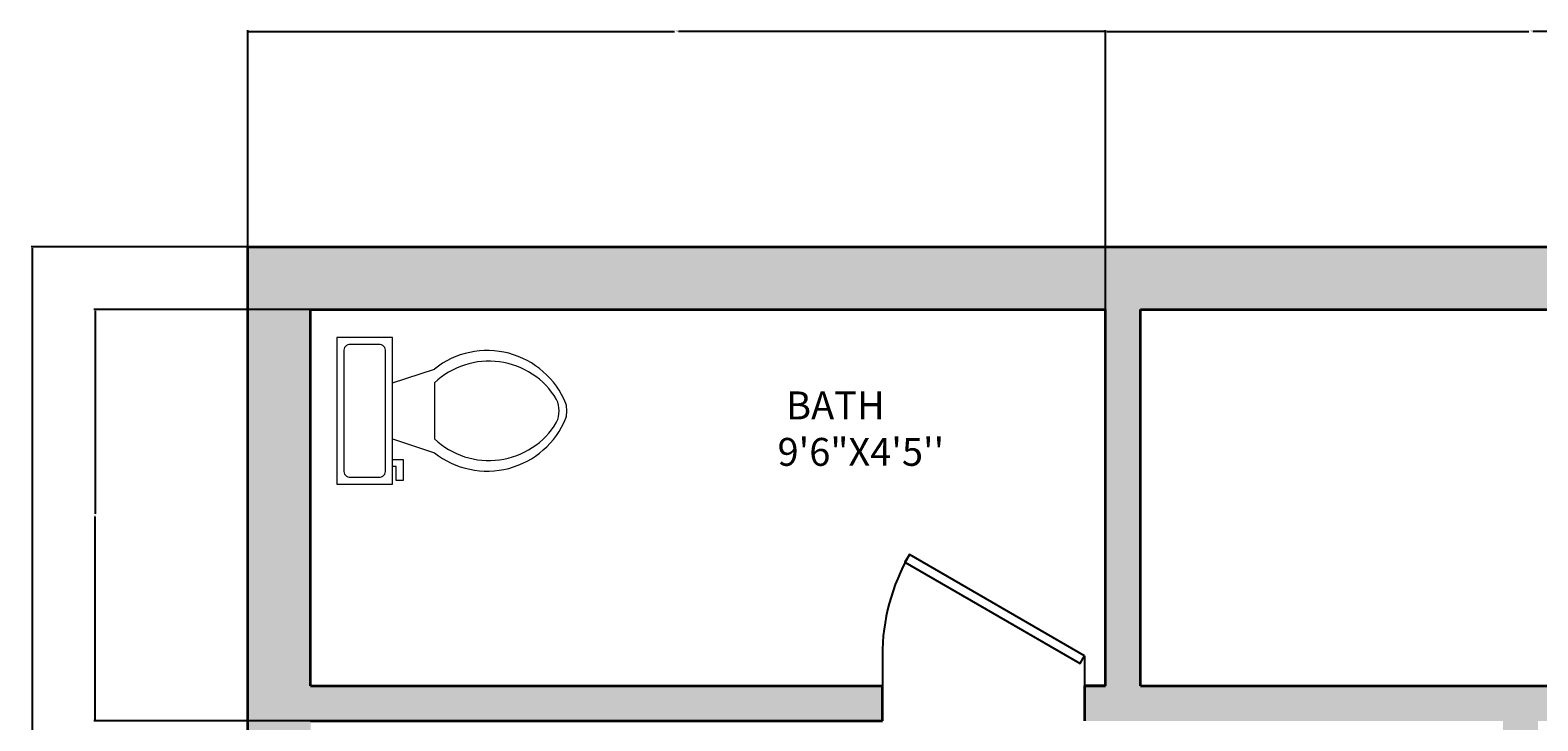
# Model space of a CAD drawing. Units: inches. Extents: x -30 to 437, y -29 to 647.
# Tile 9 of 15: x -30 to 187, y 548 to 647. Entities that reach past the tile are written whole.
import ezdxf

# ---------------------------------------------------------------- set-up
doc = ezdxf.new("R2010")
doc.units = ezdxf.units.IN
doc.header["$MEASUREMENT"] = 0
for name, color, linetype, lineweight in [('A-ANNO-DIMS', 2, 'Continuous', 18), ('A-AREA-IDEN', 7, 'Continuous', 18), ('A-WALL', 7, 'Continuous', 35), ('bathroom', 90, 'Continuous', 18), ('doors', 40, 'Continuous', 25)]:
    doc.layers.add(name, color=color, linetype=linetype, lineweight=lineweight)
doc.layers.add('A-WALL-PATT', color=251, linetype='Continuous', lineweight=13, true_color=0x636466)
doc.styles.get("Standard").update_dxf_attribs({"font": 'arial.ttf'})
doc.dimstyles.get("Standard").update_dxf_attribs({"dimtxt": 0.18, "dimasz": 0.18, "dimexe": 0.18, "dimexo": 0.0625, "dimgap": 0.09, "dimtad": 0, "dimtih": 1, "dimtoh": 1, "dimdec": 4, "dimzin": 0, "dimdsep": 46, "dimtxsty": 'Standard', "dimcen": 0.09, "dimadec": 0, "dimazin": 0, "dimtfac": 1, "dimtdec": 4, "dimtofl": 0, "dimtmove": 0, "dimatfit": 3, "dimfxl": 1, "dimtolj": 1, "dimtzin": 0, "dimarcsym": 0})

# ---------------------------------------------------------------- blocks, each defined once
blk = doc.blocks.new('Toilet - top')
for p, q in [((9.5, -6), (9.5, -2)), ((-10, -8.5), (-8, -8.5)), ((-10, -9.5), (-10, -8.5)), ((-8, -8.5), (-8, -8)), ((-7, -8), (-7, -9.5)), ((-4, -8), (-6, -14)), ((4, -8), (6, -14)), ((-7, -9.5), (-10, -9.5)), ((4, -14), (-4, -14))]:
    blk.add_line(p, q)
blk.add_lwpolyline([(10.5, -8), (10.5, 0), (-10.5, 0), (-10.5, -8)], close=True)
for points in [[(-9.5, -2), (-9.5, -6)], [(8.5, -1), (-8.5, -1)], [(-8.5, -7), (8.5, -7)]]:
    blk.add_lwpolyline(points)
for centre, radius, start, end in [((-8.62, -1.88), 0.884, 81.8699, 188.1301), ((8.62, -1.88), 0.884, 351.8699, 98.1301), ((-8.62, -6.12), 0.884, 171.8699, 278.1301), ((8.62, -6.12), 0.884, 261.8699, 8.1301), ((3.52, -21.58), 12.17, 141.4691, 247.9714), ((4.2, -21.82), 11.33, 136.3677, 238.9468), ((-3.52, -21.58), 12.17, 292.0284, 38.5307), ((-4.2, -21.82), 11.33, 301.053, 43.6321), ((0, -27.88), 4, 245.7318, 294.2682), ((0, -29), 4, 254.8605, 285.1395)]:
    blk.add_arc(centre, radius, start, end)
blk = doc.blocks.new('*U7')
for p, q in [((0, 0), (0, 6)), ((40, 0), (40, 6))]:
    blk.add_line(p, q)
blk.add_lwpolyline([(0, 0), (34.64, -20), (35.52, -18.48), (0.87, 1.52)], close=True)
blk.add_arc((0, 0), 40, 330, 0)
blk = doc.blocks.new('*D26')
at = {"layer": 'A-ANNO-DIMS', "color": 0, "lineweight": -2, "transparency": 16777216}
for p, q in [((1.61, 615.55), (-29.41, 615.55)), ((-29.23, 615.37), (-29.23, 308.98)), ((-29.23, 2.23), (-29.23, 308.62)), ((1.61, 2.05), (-29.41, 2.05))]:
    blk.add_line(p, q, dxfattribs=at)
at = {"layer": 'A-ANNO-DIMS', "color": 0, "transparency": 16777216}
for points in [[(-29.26, 615.37), (-29.2, 615.37), (-29.23, 615.55)], [(-29.26, 2.23), (-29.2, 2.23), (-29.23, 2.05)]]:
    blk.add_solid(points, dxfattribs=at)
at = {"layer": 'Defpoints', "color": 0, "transparency": 16777216}
for p in [(-29.23, 615.55), (1.67, 615.55), (1.67, 2.05)]:
    blk.add_point(p, dxfattribs=at)
at = {"layer": 'A-ANNO-DIMS', "color": 0, "transparency": 16777216, "insert": (-29.23, 308.8), "char_height": 0.18, "attachment_point": 5}
blk.add_mtext('\\A1;613.5', dxfattribs=at)
blk = doc.blocks.new('*D27')
at = {"layer": 'A-ANNO-DIMS', "color": 0, "lineweight": -2, "transparency": 16777216}
for p, q in [((1.67, 615.61), (1.67, 646.63)), ((124.67, 606.61), (124.67, 646.63)), ((1.85, 646.45), (62.89, 646.45)), ((124.49, 646.45), (63.45, 646.45))]:
    blk.add_line(p, q, dxfattribs=at)
at = {"layer": 'A-ANNO-DIMS', "color": 0, "transparency": 16777216}
for points in [[(1.85, 646.48), (1.85, 646.42), (1.67, 646.45)], [(124.49, 646.48), (124.49, 646.42), (124.67, 646.45)]]:
    blk.add_solid(points, dxfattribs=at)
at = {"layer": 'Defpoints', "color": 0, "transparency": 16777216}
for p in [(124.67, 646.45), (1.67, 615.55), (124.67, 606.55)]:
    blk.add_point(p, dxfattribs=at)
at = {"layer": 'A-ANNO-DIMS', "color": 0, "transparency": 16777216, "insert": (63.17, 646.45), "char_height": 0.18, "attachment_point": 5}
blk.add_mtext('\\A1;123', dxfattribs=at)
blk = doc.blocks.new('*D28')
at = {"layer": 'A-ANNO-DIMS', "color": 0, "lineweight": -2, "transparency": 16777216}
for p, q in [((124.67, 606.61), (124.67, 646.63)), ((246.67, 606.61), (246.67, 646.63)), ((124.85, 646.45), (185.39, 646.45)), ((246.49, 646.45), (185.95, 646.45))]:
    blk.add_line(p, q, dxfattribs=at)
at = {"layer": 'A-ANNO-DIMS', "color": 0, "transparency": 16777216}
for points in [[(124.85, 646.48), (124.85, 646.42), (124.67, 646.45)], [(246.49, 646.48), (246.49, 646.42), (246.67, 646.45)]]:
    blk.add_solid(points, dxfattribs=at)
at = {"layer": 'Defpoints', "color": 0, "transparency": 16777216}
for p in [(246.67, 646.45), (124.67, 606.55), (246.67, 606.55)]:
    blk.add_point(p, dxfattribs=at)
at = {"layer": 'A-ANNO-DIMS', "color": 0, "transparency": 16777216, "insert": (185.67, 646.45), "char_height": 0.18, "attachment_point": 5}
blk.add_mtext('\\A1;122', dxfattribs=at)
blk = doc.blocks.new('*D34')
at = {"layer": 'A-ANNO-DIMS', "color": 0, "lineweight": -2, "transparency": 16777216}
for p, q in [((10.61, 606.55), (-20.41, 606.55)), ((-20.23, 606.37), (-20.23, 577.23)), ((-20.23, 547.73), (-20.23, 576.87)), ((10.61, 547.55), (-20.41, 547.55))]:
    blk.add_line(p, q, dxfattribs=at)
at = {"layer": 'A-ANNO-DIMS', "color": 0, "transparency": 16777216}
for points in [[(-20.26, 606.37), (-20.2, 606.37), (-20.23, 606.55)], [(-20.26, 547.73), (-20.2, 547.73), (-20.23, 547.55)]]:
    blk.add_solid(points, dxfattribs=at)
at = {"layer": 'Defpoints', "color": 0, "transparency": 16777216}
for p in [(-20.23, 606.55), (10.67, 606.55), (10.67, 547.55)]:
    blk.add_point(p, dxfattribs=at)
at = {"layer": 'A-ANNO-DIMS', "color": 0, "transparency": 16777216, "insert": (-20.23, 577.05), "char_height": 0.18, "attachment_point": 5}
blk.add_mtext('\\A1;59', dxfattribs=at)

msp = doc.modelspace()

# ---------------------------------------------------------------- hatches: boundary and pattern name
at = {"layer": 'A-WALL-PATT'}
h = msp.add_hatch(color=256, dxfattribs=at)
h.dxf.hatch_style = 1
h.paths.add_polyline_path([(393.6054, 183.2352), (369.6054, 183.2352), (369.6054, 213.2352), (393.6054, 213.2352), (393.6054, 207.2352), (394.6054, 207.2352), (394.6054, 211.2352), (395.6054, 211.2352), (395.6054, 185.2352), (394.6054, 185.2352), (394.6054, 189.2352), (393.6054, 189.2352)], flags=0)
h.paths.add_polyline_path([(384.6054, 189.2352, -1), (390.6054, 189.2352, -1)], flags=0)
h.paths.add_polyline_path([(385.6054, 189.2352, -1), (389.6054, 189.2352, -1)], flags=0)
h.paths.add_polyline_path([(374.6054, 189.2352, -1), (382.6054, 189.2352, -1)], flags=0)
h.paths.add_polyline_path([(386.6054, 189.2352, -1), (388.6054, 189.2352, -1)], flags=0)
h.paths.add_polyline_path([(375.6054, 189.2352, -1), (381.6054, 189.2352, -1)], flags=0)
h.paths.add_polyline_path([(376.6054, 189.2352, -1), (380.6054, 189.2352, -1)], flags=0)
h.paths.add_polyline_path([(377.6054, 189.2352, -1), (379.6054, 189.2352, -1)], flags=0)
h.paths.add_polyline_path([(390.6054, 195.2352), (374.6054, 195.2352), (374.6054, 201.2352), (390.6054, 201.2352)], flags=0)
h.paths.add_polyline_path([(389.6054, 196.2352), (375.6054, 196.2352), (375.6054, 200.2352), (389.6054, 200.2352)], flags=0)
h.paths.add_polyline_path([(383.6054, 207.2352, -1), (391.6054, 207.2352, -1)], flags=0)
h.paths.add_polyline_path([(384.6054, 207.2352, -1), (390.6054, 207.2352, -1)], flags=0)
h.paths.add_polyline_path([(385.6054, 207.2352, -1), (389.6054, 207.2352, -1)], flags=0)
h.paths.add_polyline_path([(386.6054, 207.2352, -1), (388.6054, 207.2352, -1)], flags=0)
h.paths.add_polyline_path([(375.6054, 207.2352, -1), (381.6054, 207.2352, -1)], flags=0)
h.paths.add_polyline_path([(376.6054, 207.2352, -1), (380.6054, 207.2352, -1)], flags=0)
h.paths.add_polyline_path([(377.6054, 207.2352, -1), (379.6054, 207.2352, -1)], flags=0)
h.paths.add_polyline_path([(305.5437, 160.3663, -0.41421356), (304.0437, 158.8663), (271.0437, 158.8663, -0.41421356), (269.5437, 160.3663), (269.5437, 178.3663, -0.41421356), (271.0437, 179.8663), (304.0437, 179.8663, -0.41421356), (305.5437, 178.3663)], flags=0)
h.paths.add_polyline_path([(304.0437, 165.3663, -0.41421356), (303.0437, 164.3663), (289.2937, 164.3663, -0.41421356), (288.2937, 165.3663), (288.2937, 177.3663, -0.41421356), (289.2937, 178.3663), (303.0437, 178.3663, -0.41421356), (304.0437, 177.3663)], flags=0)
h.paths.add_polyline_path([(296.5437, 171.3663, -1), (295.5437, 171.3663, -1)], flags=0)
h.paths.add_polyline_path([(286.7937, 165.3663, -0.41421356), (285.7937, 164.3663), (272.0437, 164.3663, -0.41421356), (271.0437, 165.3663), (271.0437, 177.3663, -0.41421356), (272.0437, 178.3663), (285.7937, 178.3663, -0.41421356), (286.7937, 177.3663)], flags=0)
h.paths.add_polyline_path([(279.5437, 171.3663, -1), (278.5437, 171.3663, -1)], flags=0)
h.paths.add_polyline_path([(360.6737, 290.5474), (360.6737, 300.5474), (396.6737, 300.5474), (396.6737, 290.5474)], flags=0)
h.paths.add_polyline_path([(259.6737, 124.5474), (259.6737, 114.5474), (171.6737, 114.5474), (171.6737, 124.5474)], flags=0)
h.paths.add_polyline_path([(288.0737, 215.3705), (286.7097, 214.583), (268.7097, 245.7599), (270.0737, 246.5474)], flags=0)
h.paths.add_polyline_path([(259.6737, 168.5474), (256.6737, 168.5474), (256.6737, 173.5474), (256.6737, 179.0224), (255.8753, 177.6395), (224.2956, 195.872, 0.12053744), (220.1737, 179.0224, 0.12053744), (216.0518, 195.872), (184.4721, 177.6395), (183.6737, 179.0224), (215.2836, 197.2724), (216.0821, 195.8895), (216.0518, 195.872, -0.12053744), (220.1737, 179.0224, -0.12053744), (224.2956, 195.872), (224.2653, 195.8895), (225.0638, 197.2724), (256.6737, 179.0224), (256.6737, 173.5474), (259.6737, 173.5474)], flags=0)
h.paths.add_polyline_path([(386.7943, 325.4601), (372.6871, 325.4601), (372.6871, 339.5673), (386.7943, 339.5673)], flags=0)
h.paths.add_polyline_path([(359.5875, 343.7429), (357.7905, 343.7429), (357.7905, 327.9179), (359.3933, 327.9179, 0.41420885), (361.5302, 330.0549), (361.5302, 341.8434, 0.41436161)], flags=0)
h.paths.add_polyline_path([(341.7887, 323.1235, -0.11921667), (340.7839, 323.1235)], flags=0)
h.paths.add_polyline_path([(379.6332, 328.8632), (379.6332, 332.2699), (376.0992, 332.2699, 0.39427733)], flags=0)
h.paths.add_polyline_path([(375.5299, 332.459, -1), (383.8511, 332.459, -1)], flags=0)
h.paths.add_polyline_path([(388.9363, 344.7425), (372.5309, 344.7425, -0.41421356), (370.394, 346.8794), (370.394, 347.5594, -0.39085173), (372.3472, 349.7005, -0.43951011), (370.394, 351.4933), (370.394, 365.1894, -0.40305452), (372.2191, 367.1298, -0.41839453), (370.394, 368.9291), (370.394, 382.6251, -0.40885826), (372.2519, 384.5722, -0.42377324), (370.394, 386.3707), (370.394, 400.0667, -0.38660687), (372.1327, 402.0094), (372.531, 402.0094, -0.41421834), (370.394, 404.1464), (370.394, 404.7778, -0.41420891), (372.5309, 406.9147), (388.9363, 406.9147, -0.41421821), (391.0733, 404.7778), (391.0733, 346.8794, -0.41421356)], flags=0)
edge = h.paths.add_edge_path(flags=0)
edge.add_spline(control_points=[(349.3585, 363.204), (349.0859, 363.204), (348.8133, 363.2227), (348.2712, 363.2973), (348.0016, 363.3531), (347.3533, 363.5328), (346.9776, 363.6755), (346.2445, 364.0308), (345.887, 364.2432), (345.1953, 364.7329), (344.8611, 365.0101), (344.2197, 365.6237), (343.9125, 365.9603), (343.211, 366.8336), (342.8313, 367.3965), (342.1401, 368.6117), (341.8286, 369.2641), (341.2807, 370.64), (341.0443, 371.3636), (340.6522, 372.8619), (340.4964, 373.6367), (340.2695, 375.2158), (340.1983, 376.0203), (340.142, 377.6365), (340.157, 378.4483), (340.2729, 380.0567), (340.3738, 380.8533), (340.6589, 382.4093), (340.8432, 383.1686), (341.2906, 384.629), (341.5538, 385.3301), (342.1531, 386.6544), (342.4891, 387.2776), (343.2266, 388.4288), (343.6281, 388.9567), (344.4879, 389.9012), (344.9463, 390.3178), (345.7981, 390.9428), (346.182, 391.1771), (346.9712, 391.5648), (347.3766, 391.7182), (348.2004, 391.9387), (348.6189, 392.0058), (349.4588, 392.0508), (349.8801, 392.0288), (350.7146, 391.8966), (351.1278, 391.7865), (351.9366, 391.4822), (352.3323, 391.2882), (353.0989, 390.8223), (353.4699, 390.5504), (354.1819, 389.9355), (354.5229, 389.5924), (355.1706, 388.8418), (355.4772, 388.4343), (356.1315, 387.4422), (356.4671, 386.8397), (357.0692, 385.5581), (357.3356, 384.879), (357.7933, 383.4624), (357.9846, 382.725), (358.2875, 381.2112), (358.3992, 380.4349), (358.5404, 378.8643), (358.5699, 378.0699), (358.546, 376.4841), (358.4926, 375.6928), (358.3042, 374.1343), (358.1692, 373.3672), (357.8207, 371.8774), (357.6072, 371.1549), (357.1067, 369.7735), (356.8196, 369.1148), (356.1782, 367.8787), (355.8238, 367.3013), (355.0551, 366.244), (354.6408, 365.7641), (353.7607, 364.9161), (353.2948, 364.5481), (352.445, 364.0149), (352.0701, 363.822), (351.3034, 363.5117), (350.9116, 363.3943), (350.1325, 363.2418), (349.7455, 363.204), (349.3585, 363.204)], knot_values=[3.14159265, 3.14159265, 3.14159265, 3.14159265, 3.22691715, 3.22691715, 3.31224165, 3.31224165, 3.43426671, 3.43426671, 3.55629177, 3.55629177, 3.67831683, 3.67831683, 3.8003419, 3.8003419, 3.97157384, 3.97157384, 4.14280577, 4.14280577, 4.31403771, 4.31403771, 4.48526965, 4.48526965, 4.65650159, 4.65650159, 4.82773353, 4.82773353, 4.99896547, 4.99896547, 5.1701974, 5.1701974, 5.34142934, 5.34142934, 5.51266128, 5.51266128, 5.68389322, 5.68389322, 5.85512516, 5.85512516, 5.98669107, 5.98669107, 6.11825699, 6.11825699, 6.24982291, 6.24982291, 6.38138882, 6.38138882, 6.51295474, 6.51295474, 6.64452065, 6.64452065, 6.77608657, 6.77608657, 6.90765249, 6.90765249, 7.0392184, 7.0392184, 7.20701563, 7.20701563, 7.37481286, 7.37481286, 7.54261009, 7.54261009, 7.71040732, 7.71040732, 7.87820455, 7.87820455, 8.04600178, 8.04600178, 8.21379901, 8.21379901, 8.38159624, 8.38159624, 8.54939347, 8.54939347, 8.7171907, 8.7171907, 8.88498794, 8.88498794, 9.05278517, 9.05278517, 9.17820699, 9.17820699, 9.30362881, 9.30362881, 9.42477796, 9.42477796, 9.42477796, 9.42477796], degree=3, periodic=0)
edge.add_line((341.1696, 384.3006), (341.2012, 384.2808))
edge = h.paths.add_edge_path(flags=0)
edge.add_line((344.3353, 388.7801), (344.317, 388.7915))
edge.add_ellipse((349.3585, 377.6204), major_axis=(0, -13.7895), ratio=0.62186025, start_angle=-244.867444, end_angle=-124.769923)
h.paths.add_polyline_path([(163.6737, 163.1474), (132.4968, 145.1474), (131.7093, 146.5114), (162.8862, 164.5114)], flags=0)
h.paths.add_polyline_path([(366.4355, 409.0896, -0.41423669), (364.2985, 406.9525, -0.4913499), (361.5302, 408.8973), (361.5302, 420.6405, 0.41421356), (359.3932, 422.7775), (357.7905, 422.7775), (357.7905, 406.9525), (359.6317, 406.9525, 0.42741026), (361.5332, 408.9757, 0.39869469), (363.6672, 406.9525, 0.51958103), (366.4355, 409.0895)], flags=0)
h.paths.add_polyline_path([(386.7943, 410.9671), (372.6871, 410.9671), (372.6871, 425.0742), (386.7943, 425.0742)], flags=0)
h.paths.add_polyline_path([(379.6332, 414.3701), (379.6332, 417.7768), (376.0992, 417.7768, 0.39427733)], flags=0)
h.paths.add_polyline_path([(375.5299, 417.966, -1), (383.8511, 417.966, -1)], flags=0)
h.paths.add_polyline_path([(150.0377, 351.583), (148.6737, 352.3705), (166.6737, 383.5474), (168.0377, 382.7599)], flags=0)
h.paths.add_polyline_path([(91.6737, 234.1974), (66.559, 219.6974), (65.9246, 220.7962), (91.0393, 235.2962)], flags=0)
h.paths.add_polyline_path([(255.4612, 443.5834), (254.6737, 444.9474), (285.8506, 462.9474), (286.6381, 461.5834)], flags=0)
h.paths.add_polyline_path([(176.2737, 394.5474), (158.2737, 425.7243), (159.6377, 426.5118), (177.6377, 395.3349)], flags=0)
h.paths.add_polyline_path([(243.6737, 439.5474), (243.0393, 438.4486), (217.9246, 452.9486), (218.559, 454.0474)], flags=0)
h.paths.add_polyline_path([(38.1264, 269.8429), (40.2408, 269.8429), (40.2408, 270.3508), (38.1264, 270.3508)], flags=0)
h.paths.add_polyline_path([(75.7157, 289.9439), (40.2408, 289.9439), (38.1264, 289.6524), (40.2408, 289.6524)], flags=0)
h.paths.add_polyline_path([(75.7157, 270.0846), (77.6447, 270.0846), (77.6697, 270.1626), (75.7175, 270.1626)], flags=0)
h.paths.add_polyline_path([(80.5373, 293.3002), (33.0467, 293.3002), (13.5054, 293.3002), (13.5054, 351.9244), (29.7898, 351.9244), (80.5373, 351.9244)], flags=0)
h.paths.add_polyline_path([(46.0261, 212.466, -0.50131678), (27.1651, 207.5106), (21.165, 209.5107), (21.165, 206.5107), (22.665, 206.5107), (22.665, 203.5107), (21.165, 203.5107), (21.165, 203.0107), (13.165, 203.0107), (13.165, 224.0107), (21.165, 224.0107), (21.165, 217.5107), (27.1649, 219.5106, -0.50132349), (46.0261, 214.5554, -0.13289091)], flags=0)
h.paths.add_polyline_path([(44.688, 211.8666, -0.48007965), (27.165, 209.5107), (27.165, 217.5107, -0.4800795), (44.688, 215.1547, -0.21500378)], flags=0)
h.paths.add_polyline_path([(19.415, 204.0107), (15.165, 204.0107, -0.41421356), (14.165, 204.7607), (14.165, 222.0107, -0.41421356), (14.915, 223.0107), (19.165, 223.0107, -0.41421356), (20.165, 222.2607), (20.165, 205.0107, -0.41421356)], flags=0)
h.paths.add_polyline_path([(32.7608, 269.0719), (31.8439, 269.0719), (31.8439, 268.6134), (13.5054, 268.6134), (13.5054, 291.5366), (31.8439, 291.5366), (32.7608, 291.0781), (32.7608, 280.9919, -1), (32.7608, 279.1581)], flags=0)
h.paths.add_polyline_path([(40.2408, 360.1436), (38.1264, 360.1436), (38.1264, 359.6357), (40.2408, 359.6357)], flags=0)
h.paths.add_polyline_path([(75.7157, 355.2807), (40.2408, 355.2807), (38.1264, 355.5722), (40.2408, 355.5722), (40.2408, 355.2807), (75.7157, 355.2807), (75.7157, 375.5982), (40.2408, 375.5982), (38.1264, 375.3817), (40.2408, 375.3817), (40.2408, 375.5982), (75.7157, 375.5982), (77.9733, 375.062), (75.7175, 375.062), (75.7175, 374.554)], flags=0)
h.paths.add_polyline_path([(42.8174, 299.814, 0.13867074), (34.1602, 294.603), (14.8081, 294.603), (14.8081, 350.6216), (29.8539, 350.6216, 0.09822056)], flags=0)
h.paths.add_polyline_path([(15.8636, 276.7781, -0.30640166), (20.3757, 283.4499), (20.3483, 290.6726), (31.4014, 290.7146), (31.4309, 282.9124), (26.8287, 282.895, -0.26006276), (30.241, 276.7781, -1)], flags=0)
h.paths.add_polyline_path([(26.1332, 276.7781), (23.0523, 273.6972), (19.9714, 276.7781), (23.0523, 279.8589), (23.0523, 283.9209), (21.3493, 283.9145), (20.7006, 283.5219), (20.6907, 286.1226), (23.2914, 286.1325), (25.8936, 285.7522), (27.1939, 285.7572), (28.4928, 286.1522), (31.0935, 286.1621), (31.0918, 286.6172), (25.6303, 286.5965), (25.616, 290.3675), (31.0775, 290.3882), (31.0918, 286.6172), (31.1034, 283.5614), (28.5027, 283.5515), (25.9005, 283.9317), (23.0523, 283.9209), (23.0523, 279.8589)], flags=0)
h.paths.add_polyline_path([(24.0793, 276.7781, -1), (22.0253, 276.7781, -1)], flags=0)
h.paths.add_polyline_path([(35.7687, 302.2895, -0.41421356), (35.2283, 301.2726), (22.2164, 297.2909, -0.41421356), (21.1995, 297.8313), (15.7317, 315.6996, -0.41421356), (16.2721, 316.7165), (18.8554, 317.507), (15.3721, 328.8904, -0.41421356), (15.9125, 329.9073), (28.9244, 333.889, -0.41421356), (29.9414, 333.3486), (35.4091, 315.4802, -0.41421356), (34.8687, 314.4633), (32.2854, 313.6728)], flags=0)
h.paths.add_polyline_path([(361.3728, 532.6207), (302.7487, 532.6207), (302.7487, 580.1113), (302.7487, 599.6527), (361.3728, 599.6527), (361.3728, 583.3682)], flags=0)
h.paths.add_polyline_path([(370.1, 575.0316), (370.1, 572.9172), (370.6079, 572.9172), (370.6079, 575.0316)], flags=0)
h.paths.add_polyline_path([(385.0466, 537.4423), (385.0466, 572.9172), (384.8302, 575.0316), (384.8302, 572.9172)], flags=0)
h.paths.add_polyline_path([(384.5104, 535.3262), (384.5104, 537.4406), (384.0025, 537.4406), (364.7291, 537.4423), (364.7291, 572.9172), (365.0206, 575.0316), (365.0206, 572.9172), (364.7291, 572.9172), (364.7291, 537.4423), (384.5884, 537.4423), (384.5884, 535.5133)], flags=0)
h.paths.add_polyline_path([(384.5884, 535.5133), (383.4945, 535.164), (383.4945, 537.4406), (382.9866, 535.3262), (382.9866, 537.4406), (383.4945, 535.3262), (383.4945, 537.4406), (384.5884, 537.4406)], flags=0)
h.paths.add_polyline_path([(23.874, 286.8174), (21.0132, 286.8065), (21.0004, 290.1875), (23.8612, 290.1983)], flags=0)
h.paths.add_polyline_path([(242.9824, 511.1667), (234.9824, 511.1667), (234.9824, 517.6667), (228.9825, 515.6667, -0.50132349), (210.1213, 520.622, -0.13289091), (210.1213, 522.7114, -0.50131678), (228.9823, 527.6667), (234.9824, 525.6667), (234.9824, 528.6667), (233.4824, 528.6667), (233.4824, 531.6667), (234.9824, 531.6667), (234.9824, 532.1667), (242.9824, 532.1667)], flags=0)
h.paths.add_polyline_path([(236.9824, 512.1667, -0.41421356), (235.9824, 512.9167), (235.9824, 530.1667, -0.41421356), (236.7324, 531.1667), (240.9824, 531.1667, -0.41421356), (241.9824, 530.4167), (241.9824, 513.1667, -0.41421356), (241.2324, 512.1667)], flags=0)
h.paths.add_polyline_path([(279.533, 537.4423), (279.533, 535.5133), (279.6111, 535.4884), (279.6111, 537.4406)], flags=0)
h.paths.add_polyline_path([(279.2913, 575.0316), (279.2913, 572.9172), (279.7992, 572.9172), (279.7992, 575.0316)], flags=0)
h.paths.add_polyline_path([(211.4594, 520.0227, -0.21500378), (211.4594, 523.3107, -0.48007965), (228.9824, 525.6667), (228.9824, 517.6667, -0.4800795)], flags=0)
h.paths.add_polyline_path([(32.7627, 354.1465), (31.8457, 354.1465), (31.8457, 353.688), (13.5054, 353.688), (13.5054, 376.6134), (31.8457, 376.6134), (32.7627, 376.1549), (32.7627, 366.0677, -1), (32.7627, 364.2337)], flags=0)
h.paths.add_polyline_path([(15.9446, 365.1507, -1), (30.3234, 365.1507, -1)], flags=0)
h.paths.add_polyline_path([(41.213, 428.467), (43.3274, 428.467), (43.3274, 428.9749), (41.213, 428.9749)], flags=0)
h.paths.add_polyline_path([(78.8022, 448.568), (43.3274, 448.568), (41.213, 448.2765), (43.3274, 448.2765)], flags=0)
h.paths.add_polyline_path([(78.8022, 428.7087), (80.7313, 428.7087), (80.7562, 428.7868), (78.804, 428.7868)], flags=0)
h.paths.add_polyline_path([(26.2152, 365.1507), (23.134, 362.0696), (20.0529, 365.1507), (23.134, 368.2319)], flags=0)
h.paths.add_polyline_path([(24.1611, 365.1507, -1), (22.107, 365.1507, -1)], flags=0)
h.paths.add_polyline_path([(309.2625, 570.3406, 0.13867074), (304.0514, 578.9978), (304.0514, 598.3499), (360.07, 598.3499), (360.07, 583.3041, 0.09822056)], flags=0)
h.paths.add_polyline_path([(246.6737, 552.5474), (129.6737, 552.5474), (129.6737, 606.5474), (246.6737, 606.5474)], flags=16)
h.paths.add_polyline_path([(373.6822, 580.3953), (363.595, 580.3953), (363.595, 581.3123), (363.1365, 581.3123), (363.1365, 599.6527), (386.0619, 599.6527), (386.0619, 581.3123), (385.6034, 580.3953), (375.5162, 580.3953, -1)], flags=0)
h.paths.add_polyline_path([(83.6239, 451.9244), (36.1333, 451.9244), (16.5919, 451.9244), (16.5919, 510.5485), (32.8764, 510.5485), (83.6239, 510.5485)], flags=0)
h.paths.add_polyline_path([(367.4098, 590.024, -1), (381.7886, 590.024, -1)], flags=0)
h.paths.add_polyline_path([(374.5992, 586.9428), (371.518, 590.024), (374.5992, 593.1052), (377.6803, 590.024)], flags=0)
h.paths.add_polyline_path([(373.5721, 590.024, -1), (375.6262, 590.024, -1)], flags=0)
h.paths.add_polyline_path([(324.9287, 577.7489, -0.41421356), (323.9118, 578.2893), (323.1212, 580.8726), (311.7379, 577.3893, -0.41421356), (310.721, 577.9297), (306.7393, 590.9416, -0.41421356), (307.2797, 591.9585), (325.1481, 597.4263, -0.41421356), (326.165, 596.8859), (326.9555, 594.3026), (338.3388, 597.7859, -0.41421356), (339.3557, 597.2455), (343.3374, 584.2336, -0.41421356), (342.797, 583.2167)], flags=0)
h.paths.add_polyline_path([(300.5265, 580.3972), (290.4404, 580.3972, -1), (288.6065, 580.3972), (278.5203, 580.3972), (278.5203, 581.3142), (278.0619, 581.3142), (278.0619, 599.6527), (300.985, 599.6527), (300.985, 581.3142)], flags=0)
h.paths.add_polyline_path([(300.163, 581.7567), (292.3609, 581.7271), (292.3434, 586.3294, -0.75567924), (279.0378, 590.1057, -0.82536731), (292.8983, 592.7823), (300.1211, 592.8097)], flags=0)
h.paths.add_polyline_path([(299.8367, 582.0805), (296.0656, 582.0662), (293.0098, 582.0546), (292.9999, 584.6553), (293.3802, 587.2575), (293.3694, 590.1057), (289.3074, 590.1057), (286.2265, 587.0248), (283.1456, 590.1057), (286.2265, 593.1866), (289.3074, 590.1057), (293.3694, 590.1057), (293.3629, 591.8088), (292.9703, 592.4575), (295.5711, 592.4673), (295.5809, 589.8666), (295.2007, 587.2644), (295.2056, 585.9641), (295.6006, 584.6652), (295.6105, 582.0645), (296.0656, 582.0662), (296.0449, 587.5277), (299.8159, 587.542)], flags=0)
h.paths.add_polyline_path([(285.1995, 590.1057, -1), (287.2535, 590.1057, -1)], flags=0)
h.paths.add_polyline_path([(299.6467, 589.2969), (296.2658, 589.284), (296.255, 592.1448), (299.6359, 592.1576)], flags=0)
h.paths.add_polyline_path([(35.8473, 427.696), (34.9304, 427.696), (34.9304, 427.2376), (16.5919, 427.2376), (16.5919, 450.1607), (34.9304, 450.1607), (35.8473, 449.7022), (35.8473, 439.6161, -1), (35.8473, 437.7822)], flags=0)
h.paths.add_polyline_path([(18.9502, 435.4022, -0.30640166), (23.4623, 442.074), (23.4349, 449.2968), (34.4879, 449.3387), (34.5175, 441.5366), (29.9152, 441.5191, -0.26006276), (33.3275, 435.4022, -1)], flags=0)
h.paths.add_polyline_path([(29.2197, 435.4022), (26.1389, 432.3213), (23.058, 435.4022), (26.1389, 438.4831), (26.1389, 442.5451), (24.4358, 442.5386), (23.7871, 442.1461), (23.7772, 444.7468), (26.378, 444.7566), (28.9801, 444.3764), (30.2805, 444.3813), (31.5794, 444.7764), (34.1801, 444.7862), (34.1784, 445.2413), (28.7169, 445.2206), (28.7026, 448.9917), (34.164, 449.0124), (34.1784, 445.2413), (34.1899, 442.1855), (31.5892, 442.1756), (28.987, 442.5559), (26.1389, 442.5451), (26.1389, 438.4831)], flags=0)
h.paths.add_polyline_path([(27.1658, 435.4022, -1), (25.1119, 435.4022, -1)], flags=0)
h.paths.add_polyline_path([(45.904, 458.4382, 0.13867074), (37.2467, 453.2271), (17.8947, 453.2271), (17.8947, 509.2457), (32.9405, 509.2457, 0.09822056)], flags=0)
h.paths.add_polyline_path([(26.9605, 445.4415), (24.0997, 445.4307), (24.0869, 448.8116), (26.9477, 448.8225)], flags=0)
h.paths.add_polyline_path([(38.3149, 459.8967), (25.3029, 455.915, -0.41421356), (24.286, 456.4554), (18.8183, 474.3238, -0.41421356), (19.3586, 475.3407), (21.942, 476.1312), (18.4587, 487.5145, -0.41421356), (18.999, 488.5314), (32.011, 492.5131, -0.41421356), (33.0279, 491.9727), (38.4957, 474.1044, -0.41421356), (37.9553, 473.0875), (35.3719, 472.297), (38.8553, 460.9136, -0.41421356)], flags=0)
h.paths.add_polyline_path([(43.3274, 518.7678), (41.213, 518.7678), (41.213, 518.2598), (43.3274, 518.2598)], flags=0)
h.paths.add_polyline_path([(78.8022, 513.9049), (43.3274, 513.9049), (41.213, 514.1964), (43.3274, 514.1964), (43.3274, 513.9049), (78.8022, 513.9049), (78.8022, 534.2223), (43.3274, 534.2223), (41.213, 534.0059), (43.3274, 534.0059), (43.3274, 534.2223), (78.8022, 534.2223), (81.0599, 533.6861), (78.804, 533.6861), (78.804, 533.1782)], flags=0)
h.paths.add_polyline_path([(121.6737, 556.8974), (121.0393, 555.7986), (95.9246, 570.2986), (96.559, 571.3974)], flags=0)
h.paths.add_polyline_path([(35.8493, 512.7707), (34.9322, 512.7707), (34.9322, 512.3122), (16.5919, 512.3122), (16.5919, 535.2376), (34.9322, 535.2376), (35.8493, 534.7791), (35.8493, 524.6919, -1), (35.8493, 522.8579)], flags=0)
h.paths.add_polyline_path([(19.0312, 523.7749, -1), (33.41, 523.7749, -1)], flags=0)
h.paths.add_polyline_path([(26.2206, 520.6937), (23.1394, 523.7749), (26.2206, 526.8561), (29.3018, 523.7749)], flags=0)
h.paths.add_polyline_path([(25.1935, 523.7749, -1), (27.2476, 523.7749, -1)], flags=0)
h.paths.add_polyline_path([(28.4381, 586.0173), (22.438, 588.0173), (22.438, 585.0173), (23.938, 585.0173), (23.938, 582.0173), (22.438, 582.0173), (22.438, 581.5173), (14.438, 581.5173), (14.438, 602.5173), (22.438, 602.5173), (22.438, 596.0173), (28.4379, 598.0173, -0.50132349), (47.2992, 593.062, -0.13289091), (47.2992, 590.9726, -0.50131678)], flags=0)
h.paths.add_polyline_path([(28.438, 588.0174), (28.438, 596.0173, -0.4800795), (45.961, 593.6614, -0.21500378), (45.961, 590.3733, -0.48007965)], flags=0)
h.paths.add_polyline_path([(20.688, 582.5173), (16.438, 582.5173, -0.41421356), (15.438, 583.2673), (15.438, 600.5173, -0.41421356), (16.188, 601.5173), (20.438, 601.5173, -0.41421356), (21.438, 600.7673), (21.438, 583.5173, -0.41421356)], flags=0)
h.paths.add_polyline_path([(171.6737, 2.0474), (171.6737, 104.5474), (259.6737, 104.5474), (259.6737, 148.5474), (396.6737, 148.5474), (396.6737, 2.0474), (405.6737, 2.0474), (405.6737, 615.5474), (1.6737, 615.5474), (1.6737, 2.0474)])
h.paths.add_polyline_path([(171.6737, 104.5474), (259.6737, 104.5474), (259.6737, 210.5474), (264.6737, 210.5474), (264.6737, 153.5474), (396.6737, 153.5474), (396.6737, 249.5474), (264.6737, 249.5474), (264.6737, 246.5474), (259.6737, 246.5474), (259.6737, 254.5474), (396.6737, 254.5474), (396.6737, 434.5474), (290.6737, 434.5474), (290.6737, 439.5474), (396.6737, 439.5474), (396.6737, 606.5474), (251.6737, 606.5474), (251.6737, 439.5474), (254.6737, 439.5474), (254.6737, 434.5474), (243.6737, 434.5474), (243.6737, 439.5474), (246.6737, 439.5474), (246.6737, 547.5474), (186.6737, 547.5474), (186.6737, 439.5474), (214.6737, 439.5474), (214.6737, 434.5474), (186.6737, 434.5474), (186.6737, 430.5474), (181.6737, 430.5474), (181.6737, 547.5474), (121.6737, 547.5474), (121.6737, 552.5474), (124.6737, 552.5474), (124.6737, 606.5474), (10.6737, 606.5474), (10.6737, 552.5474), (92.6737, 552.5474), (92.6737, 547.5474), (10.6737, 547.5474), (10.6737, 391.5474), (181.6737, 391.5474), (181.6737, 394.5474), (186.6737, 394.5474), (186.6737, 386.5474), (171.6737, 386.5474), (171.6737, 383.5474), (166.6737, 383.5474), (166.6737, 386.5474), (10.6737, 386.5474), (10.6737, 238.5474), (62.6737, 238.5474), (62.6737, 233.5474), (10.6737, 233.5474), (10.6737, 173.5474), (94.6737, 173.5474), (94.6737, 233.5474), (91.6737, 233.5474), (91.6737, 238.5474), (166.6737, 238.5474), (166.6737, 347.5474), (171.6737, 347.5474), (171.6737, 233.5474), (99.6737, 233.5474), (99.6737, 173.5474), (127.6737, 173.5474), (127.6737, 168.5474), (10.6737, 168.5474), (10.6737, 11.0474), (166.6737, 11.0474), (166.6737, 168.5474), (163.6737, 168.5474), (163.6737, 173.5474), (183.6737, 173.5474), (183.6737, 168.5474), (171.6737, 168.5474)])

# ---------------------------------------------------------------- linework, layer by layer
at = {"layer": 'A-WALL'}
for p, q in [((10.6737, 606.5474), (124.6737, 606.5474)), ((10.6737, 552.5474), (10.6737, 606.5474)), ((124.6737, 552.5474), (124.6737, 606.5474)), ((129.6737, 606.5474), (246.6737, 606.5474)), ((129.6737, 552.5474), (129.6737, 606.5474)), ((10.6737, 552.5474), (92.6737, 552.5474)), ((92.6737, 547.5474), (92.6737, 552.5474)), ((121.6737, 552.5474), (124.6737, 552.5474)), ((124.6737, 552.5474), (121.6737, 552.5474)), ((121.6737, 552.5474), (121.6737, 547.5474)), ((129.6737, 552.5474), (246.6737, 552.5474)), ((10.6737, 547.5474), (92.6737, 547.5474))]:
    msp.add_line(p, q, dxfattribs=at)
msp.add_lwpolyline([(171.6737, 2.0474), (1.6737, 2.0474), (1.6737, 615.5474), (405.6737, 615.5474), (405.6737, 2.0474), (396.6737, 2.0474)], dxfattribs=at)

# ---------------------------------------------------------------- block references
at = {"layer": 'bathroom', "rotation": 90}
msp.add_blockref('Toilet - top', (14.438, 592.0173), dxfattribs=at)
at = {"layer": 'doors', "xscale": 0.725, "yscale": 0.725, "zscale": 0.725, "rotation": 180}
msp.add_blockref('*U7', (121.6737, 556.8974), dxfattribs=at)

# ---------------------------------------------------------------- texts
at = {"layer": 'A-AREA-IDEN', "insert": (77.6445, 594.7989), "char_height": 4, "attachment_point": 1}
msp.add_mtext_dynamic_manual_height_columns(' BATH\\P    9\'6"X4\'5\'\'', width=25.99481, gutter_width=1, heights=[0], dxfattribs=at)

# ---------------------------------------------------------------- dimensions: what is measured, and where the dimension line sits
at = {"layer": 'A-ANNO-DIMS'}
for base, p1, p2, picture, middle in [((124.6737, 646.4474), (1.6737, 615.5474), (124.6737, 606.5474), '*D27', (63.1737, 646.4474)), ((246.6737, 646.4474), (124.6737, 606.5474), (246.6737, 606.5474), '*D28', (185.6737, 646.4474))]:
    dim = msp.add_linear_dim(base=base, p1=p1, p2=p2, dimstyle='Standard', override={"dimdec": 0, "dimlfac": 1, "dimrnd": 0, "dimzin": 0, "dimdsep": 46, "dimlunit": 2}, dxfattribs=at)
    dim.commit()
    dim.dimension.update_dxf_attribs({"geometry": picture, "text_midpoint": middle})
for base, p1, p2, override, picture, middle in [((-29.2263, 615.5474), (1.6737, 2.0474), (1.6737, 615.5474), {"dimdec": 1, "dimlfac": 1, "dimrnd": 0, "dimzin": 0, "dimdsep": 46, "dimlunit": 2}, '*D26', (-29.2263, 308.7974)), ((-20.2263, 606.5474), (10.6737, 547.5474), (10.6737, 606.5474), {"dimdec": 0, "dimlfac": 1, "dimrnd": 0, "dimzin": 0, "dimdsep": 46, "dimlunit": 2}, '*D34', (-20.2263, 577.0474))]:
    dim = msp.add_linear_dim(base=base, p1=p1, p2=p2, angle=90, dimstyle='Standard', override=override, dxfattribs=at)
    dim.commit()
    dim.dimension.update_dxf_attribs({"geometry": picture, "text_midpoint": middle})

doc.saveas('drawing.dxf')
